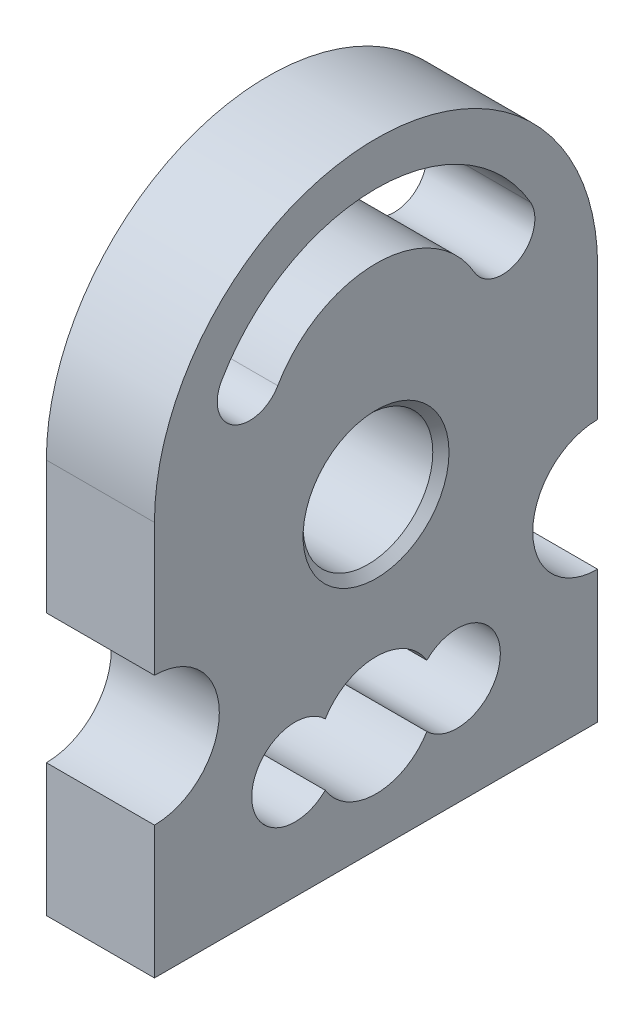
ISO-10303-21;
HEADER;
FILE_DESCRIPTION(('STEP AP214'),'2;1');
FILE_NAME('part.step','',(''),(''),'','','');
FILE_SCHEMA(('AUTOMOTIVE_DESIGN { 1 0 10303 214 1 1 1 1 }'));
ENDSEC;
DATA;
#1=APPLICATION_CONTEXT('core data for automotive mechanical design processes');
#2=APPLICATION_PROTOCOL_DEFINITION('international standard','automotive_design',2000,#1);
#3=PRODUCT_CONTEXT('',#1,'mechanical');
#4=PRODUCT('Part','Part','',(#3));
#5=PRODUCT_RELATED_PRODUCT_CATEGORY('part','',(#4));
#6=PRODUCT_DEFINITION_FORMATION('','',#4);
#7=PRODUCT_DEFINITION_CONTEXT('part definition',#1,'design');
#8=PRODUCT_DEFINITION('design','',#6,#7);
#9=PRODUCT_DEFINITION_SHAPE('','',#8);
#10=(LENGTH_UNIT() NAMED_UNIT(*) SI_UNIT(.MILLI.,.METRE.));
#11=(NAMED_UNIT(*) PLANE_ANGLE_UNIT() SI_UNIT($,.RADIAN.));
#12=(NAMED_UNIT(*) SI_UNIT($,.STERADIAN.) SOLID_ANGLE_UNIT());
#13=UNCERTAINTY_MEASURE_WITH_UNIT(LENGTH_MEASURE(1.E-05),#10,'distance_accuracy_value','');
#14=(GEOMETRIC_REPRESENTATION_CONTEXT(3) GLOBAL_UNCERTAINTY_ASSIGNED_CONTEXT((#13)) GLOBAL_UNIT_ASSIGNED_CONTEXT((#10,
#11,#12)) REPRESENTATION_CONTEXT('',''));
#15=CARTESIAN_POINT('',(0.,0.,0.));
#16=DIRECTION('',(0.,0.,1.));
#17=DIRECTION('',(1.,0.,0.));
#18=AXIS2_PLACEMENT_3D('',#15,#16,#17);
#19=CARTESIAN_POINT('',(20.,36.5,-41.));
#20=DIRECTION('',(1.,0.,0.));
#21=DIRECTION('',(0.,0.,-1.));
#22=AXIS2_PLACEMENT_3D('',#19,#20,#21);
#23=PLANE('',#22);
#24=CARTESIAN_POINT('',(20.,57.,0.));
#25=DIRECTION('',(1.,0.,0.));
#26=DIRECTION('',(0.,0.,-1.));
#27=AXIS2_PLACEMENT_3D('',#24,#25,#26);
#28=CIRCLE('',#27,13.5000000000001);
#29=CARTESIAN_POINT('',(20.,57.,-13.5000000000001));
#30=VERTEX_POINT('',#29);
#31=EDGE_CURVE('E11',#30,#30,#28,.F.);
#32=ORIENTED_EDGE('',*,*,#31,.T.);
#33=EDGE_LOOP('',(#32));
#34=FACE_BOUND('',#33,.T.);
#35=CARTESIAN_POINT('',(20.,20.,-15.));
#36=DIRECTION('',(1.,0.,0.));
#37=DIRECTION('',(0.,0.,-1.));
#38=AXIS2_PLACEMENT_3D('',#35,#36,#37);
#39=CIRCLE('',#38,8.);
#40=CARTESIAN_POINT('',(20.,14.2868572571657,-9.4));
#41=VERTEX_POINT('',#40);
#42=CARTESIAN_POINT('',(20.,25.7131427428343,-9.4));
#43=VERTEX_POINT('',#42);
#44=EDGE_CURVE('E193',#41,#43,#39,.T.);
#45=ORIENTED_EDGE('',*,*,#44,.F.);
#46=CARTESIAN_POINT('',(20.,20.,0.));
#47=DIRECTION('',(1.,0.,0.));
#48=DIRECTION('',(0.,0.,-1.));
#49=AXIS2_PLACEMENT_3D('',#46,#47,#48);
#50=CIRCLE('',#49,11.);
#51=CARTESIAN_POINT('',(20.,14.2868572571657,9.4));
#52=VERTEX_POINT('',#51);
#53=EDGE_CURVE('E192',#52,#41,#50,.T.);
#54=ORIENTED_EDGE('',*,*,#53,.F.);
#55=CARTESIAN_POINT('',(20.,20.,15.));
#56=DIRECTION('',(1.,0.,0.));
#57=DIRECTION('',(0.,0.,-1.));
#58=AXIS2_PLACEMENT_3D('',#55,#56,#57);
#59=CIRCLE('',#58,8.);
#60=CARTESIAN_POINT('',(20.,25.7131427428343,9.4));
#61=VERTEX_POINT('',#60);
#62=EDGE_CURVE('E200',#61,#52,#59,.T.);
#63=ORIENTED_EDGE('',*,*,#62,.F.);
#64=CARTESIAN_POINT('',(20.,20.,0.));
#65=DIRECTION('',(1.,0.,0.));
#66=DIRECTION('',(0.,0.,-1.));
#67=AXIS2_PLACEMENT_3D('',#64,#65,#66);
#68=CIRCLE('',#67,11.);
#69=EDGE_CURVE('E198',#43,#61,#68,.T.);
#70=ORIENTED_EDGE('',*,*,#69,.F.);
#71=EDGE_LOOP('',(#45,#54,#63,#70));
#72=FACE_BOUND('',#71,.T.);
#73=DIRECTION('',(0.,0.,-1.));
#74=VECTOR('',#73,1.);
#75=CARTESIAN_POINT('',(20.,0.,0.));
#76=LINE('',#75,#74);
#77=CARTESIAN_POINT('',(20.,0.,41.));
#78=VERTEX_POINT('',#77);
#79=CARTESIAN_POINT('',(20.,0.,-41.));
#80=VERTEX_POINT('',#79);
#81=EDGE_CURVE('E225',#78,#80,#76,.T.);
#82=ORIENTED_EDGE('',*,*,#81,.T.);
#83=DIRECTION('',(0.,1.,0.));
#84=VECTOR('',#83,1.);
#85=CARTESIAN_POINT('',(20.,24.5,-41.));
#86=LINE('',#85,#84);
#87=CARTESIAN_POINT('',(20.,24.5,-41.));
#88=VERTEX_POINT('',#87);
#89=EDGE_CURVE('E223',#80,#88,#86,.T.);
#90=ORIENTED_EDGE('',*,*,#89,.T.);
#91=CARTESIAN_POINT('',(20.,36.5,-41.));
#92=DIRECTION('',(-1.,0.,0.));
#93=DIRECTION('',(0.,0.,-1.));
#94=AXIS2_PLACEMENT_3D('',#91,#92,#93);
#95=CIRCLE('',#94,12.);
#96=CARTESIAN_POINT('',(20.,48.5,-41.));
#97=VERTEX_POINT('',#96);
#98=EDGE_CURVE('E229',#88,#97,#95,.T.);
#99=ORIENTED_EDGE('',*,*,#98,.T.);
#100=DIRECTION('',(0.,1.,0.));
#101=VECTOR('',#100,1.);
#102=CARTESIAN_POINT('',(20.,73.,-41.));
#103=LINE('',#102,#101);
#104=CARTESIAN_POINT('',(20.,73.,-41.));
#105=VERTEX_POINT('',#104);
#106=EDGE_CURVE('E228',#97,#105,#103,.T.);
#107=ORIENTED_EDGE('',*,*,#106,.T.);
#108=CARTESIAN_POINT('',(20.,73.,0.));
#109=DIRECTION('',(1.,0.,0.));
#110=DIRECTION('',(0.,0.,-1.));
#111=AXIS2_PLACEMENT_3D('',#108,#109,#110);
#112=CIRCLE('',#111,41.);
#113=CARTESIAN_POINT('',(20.,73.,41.));
#114=VERTEX_POINT('',#113);
#115=EDGE_CURVE('E235',#105,#114,#112,.T.);
#116=ORIENTED_EDGE('',*,*,#115,.T.);
#117=DIRECTION('',(0.,-1.,0.));
#118=VECTOR('',#117,1.);
#119=CARTESIAN_POINT('',(20.,73.,41.));
#120=LINE('',#119,#118);
#121=CARTESIAN_POINT('',(20.,48.5,41.));
#122=VERTEX_POINT('',#121);
#123=EDGE_CURVE('E234',#114,#122,#120,.T.);
#124=ORIENTED_EDGE('',*,*,#123,.T.);
#125=CARTESIAN_POINT('',(20.,36.5,41.));
#126=DIRECTION('',(-1.,0.,0.));
#127=DIRECTION('',(0.,0.,-1.));
#128=AXIS2_PLACEMENT_3D('',#125,#126,#127);
#129=CIRCLE('',#128,12.);
#130=CARTESIAN_POINT('',(20.,24.5,41.));
#131=VERTEX_POINT('',#130);
#132=EDGE_CURVE('E237',#122,#131,#129,.T.);
#133=ORIENTED_EDGE('',*,*,#132,.T.);
#134=DIRECTION('',(0.,-1.,0.));
#135=VECTOR('',#134,1.);
#136=CARTESIAN_POINT('',(20.,24.5,41.));
#137=LINE('',#136,#135);
#138=EDGE_CURVE('E236',#131,#78,#137,.T.);
#139=ORIENTED_EDGE('',*,*,#138,.T.);
#140=EDGE_LOOP('',(#82,#90,#99,#107,#116,#124,#133,#139));
#141=FACE_BOUND('',#140,.T.);
#142=CARTESIAN_POINT('',(20.,73.,0.));
#143=DIRECTION('',(1.,0.,0.));
#144=DIRECTION('',(0.,0.,-1.));
#145=AXIS2_PLACEMENT_3D('',#142,#143,#144);
#146=CIRCLE('',#145,33.);
#147=CARTESIAN_POINT('',(20.,89.4999999999999,-28.5788383248865));
#148=VERTEX_POINT('',#147);
#149=CARTESIAN_POINT('',(20.,89.4999999999999,28.5788383248865));
#150=VERTEX_POINT('',#149);
#151=EDGE_CURVE('E162',#148,#150,#146,.T.);
#152=ORIENTED_EDGE('',*,*,#151,.F.);
#153=CARTESIAN_POINT('',(20.,86.4999999999999,-23.3826859021799));
#154=DIRECTION('',(1.,0.,0.));
#155=DIRECTION('',(0.,0.,-1.));
#156=AXIS2_PLACEMENT_3D('',#153,#154,#155);
#157=CIRCLE('',#156,6.);
#158=CARTESIAN_POINT('',(20.,83.4999999999999,-18.1865334794732));
#159=VERTEX_POINT('',#158);
#160=EDGE_CURVE('E154',#159,#148,#157,.T.);
#161=ORIENTED_EDGE('',*,*,#160,.F.);
#162=CARTESIAN_POINT('',(20.,73.,0.));
#163=DIRECTION('',(-1.,0.,0.));
#164=DIRECTION('',(0.,0.,-1.));
#165=AXIS2_PLACEMENT_3D('',#162,#163,#164);
#166=CIRCLE('',#165,21.);
#167=CARTESIAN_POINT('',(20.,83.4999999999999,18.1865334794732));
#168=VERTEX_POINT('',#167);
#169=EDGE_CURVE('E180',#168,#159,#166,.T.);
#170=ORIENTED_EDGE('',*,*,#169,.F.);
#171=CARTESIAN_POINT('',(20.,86.4999999999999,23.3826859021799));
#172=DIRECTION('',(1.,0.,0.));
#173=DIRECTION('',(0.,0.,-1.));
#174=AXIS2_PLACEMENT_3D('',#171,#172,#173);
#175=CIRCLE('',#174,6.);
#176=EDGE_CURVE('E173',#150,#168,#175,.T.);
#177=ORIENTED_EDGE('',*,*,#176,.F.);
#178=EDGE_LOOP('',(#152,#161,#170,#177));
#179=FACE_BOUND('',#178,.T.);
#180=ADVANCED_FACE('F41',(#34,#72,#141,#179),#23,.T.);
#181=CARTESIAN_POINT('',(0.,36.5,-41.));
#182=DIRECTION('',(1.,0.,0.));
#183=DIRECTION('',(0.,0.,-1.));
#184=AXIS2_PLACEMENT_3D('',#181,#182,#183);
#185=PLANE('',#184);
#186=CARTESIAN_POINT('',(0.,57.,0.));
#187=DIRECTION('',(1.,0.,0.));
#188=DIRECTION('',(0.,0.,-1.));
#189=AXIS2_PLACEMENT_3D('',#186,#187,#188);
#190=CIRCLE('',#189,13.5);
#191=CARTESIAN_POINT('',(0.,57.,-13.5));
#192=VERTEX_POINT('',#191);
#193=EDGE_CURVE('E276',#192,#192,#190,.T.);
#194=ORIENTED_EDGE('',*,*,#193,.T.);
#195=EDGE_LOOP('',(#194));
#196=FACE_BOUND('',#195,.T.);
#197=CARTESIAN_POINT('',(0.,20.,0.));
#198=DIRECTION('',(1.,0.,0.));
#199=DIRECTION('',(0.,0.,-1.));
#200=AXIS2_PLACEMENT_3D('',#197,#198,#199);
#201=CIRCLE('',#200,11.);
#202=CARTESIAN_POINT('',(0.,14.2868572571657,9.4));
#203=VERTEX_POINT('',#202);
#204=CARTESIAN_POINT('',(0.,14.2868572571657,-9.4));
#205=VERTEX_POINT('',#204);
#206=EDGE_CURVE('E172',#203,#205,#201,.T.);
#207=ORIENTED_EDGE('',*,*,#206,.T.);
#208=CARTESIAN_POINT('',(0.,20.,-15.));
#209=DIRECTION('',(1.,0.,0.));
#210=DIRECTION('',(0.,0.,-1.));
#211=AXIS2_PLACEMENT_3D('',#208,#209,#210);
#212=CIRCLE('',#211,8.);
#213=CARTESIAN_POINT('',(0.,25.7131427428343,-9.4));
#214=VERTEX_POINT('',#213);
#215=EDGE_CURVE('E204',#205,#214,#212,.T.);
#216=ORIENTED_EDGE('',*,*,#215,.T.);
#217=CARTESIAN_POINT('',(0.,20.,0.));
#218=DIRECTION('',(1.,0.,0.));
#219=DIRECTION('',(0.,0.,-1.));
#220=AXIS2_PLACEMENT_3D('',#217,#218,#219);
#221=CIRCLE('',#220,11.);
#222=CARTESIAN_POINT('',(0.,25.7131427428343,9.4));
#223=VERTEX_POINT('',#222);
#224=EDGE_CURVE('E210',#214,#223,#221,.T.);
#225=ORIENTED_EDGE('',*,*,#224,.T.);
#226=CARTESIAN_POINT('',(0.,20.,15.));
#227=DIRECTION('',(1.,0.,0.));
#228=DIRECTION('',(0.,0.,-1.));
#229=AXIS2_PLACEMENT_3D('',#226,#227,#228);
#230=CIRCLE('',#229,8.);
#231=EDGE_CURVE('E194',#223,#203,#230,.T.);
#232=ORIENTED_EDGE('',*,*,#231,.T.);
#233=EDGE_LOOP('',(#207,#216,#225,#232));
#234=FACE_BOUND('',#233,.T.);
#235=DIRECTION('',(0.,1.,0.));
#236=VECTOR('',#235,1.);
#237=CARTESIAN_POINT('',(0.,24.5,-41.));
#238=LINE('',#237,#236);
#239=CARTESIAN_POINT('',(0.,0.,-41.));
#240=VERTEX_POINT('',#239);
#241=CARTESIAN_POINT('',(0.,24.5,-41.));
#242=VERTEX_POINT('',#241);
#243=EDGE_CURVE('E222',#240,#242,#238,.T.);
#244=ORIENTED_EDGE('',*,*,#243,.F.);
#245=DIRECTION('',(0.,0.,-1.));
#246=VECTOR('',#245,1.);
#247=CARTESIAN_POINT('',(0.,0.,0.));
#248=LINE('',#247,#246);
#249=CARTESIAN_POINT('',(0.,0.,41.));
#250=VERTEX_POINT('',#249);
#251=EDGE_CURVE('E227',#250,#240,#248,.T.);
#252=ORIENTED_EDGE('',*,*,#251,.F.);
#253=DIRECTION('',(0.,-1.,0.));
#254=VECTOR('',#253,1.);
#255=CARTESIAN_POINT('',(0.,24.5,41.));
#256=LINE('',#255,#254);
#257=CARTESIAN_POINT('',(0.,24.5,41.));
#258=VERTEX_POINT('',#257);
#259=EDGE_CURVE('E251',#258,#250,#256,.T.);
#260=ORIENTED_EDGE('',*,*,#259,.F.);
#261=CARTESIAN_POINT('',(0.,36.5,41.));
#262=DIRECTION('',(-1.,0.,0.));
#263=DIRECTION('',(0.,0.,-1.));
#264=AXIS2_PLACEMENT_3D('',#261,#262,#263);
#265=CIRCLE('',#264,12.);
#266=CARTESIAN_POINT('',(0.,48.5,41.));
#267=VERTEX_POINT('',#266);
#268=EDGE_CURVE('E253',#267,#258,#265,.T.);
#269=ORIENTED_EDGE('',*,*,#268,.F.);
#270=DIRECTION('',(0.,-1.,0.));
#271=VECTOR('',#270,1.);
#272=CARTESIAN_POINT('',(0.,73.,41.));
#273=LINE('',#272,#271);
#274=CARTESIAN_POINT('',(0.,73.,41.));
#275=VERTEX_POINT('',#274);
#276=EDGE_CURVE('E249',#275,#267,#273,.T.);
#277=ORIENTED_EDGE('',*,*,#276,.F.);
#278=CARTESIAN_POINT('',(0.,73.,0.));
#279=DIRECTION('',(1.,0.,0.));
#280=DIRECTION('',(0.,0.,-1.));
#281=AXIS2_PLACEMENT_3D('',#278,#279,#280);
#282=CIRCLE('',#281,41.);
#283=CARTESIAN_POINT('',(0.,73.,-41.));
#284=VERTEX_POINT('',#283);
#285=EDGE_CURVE('E250',#284,#275,#282,.T.);
#286=ORIENTED_EDGE('',*,*,#285,.F.);
#287=DIRECTION('',(0.,1.,0.));
#288=VECTOR('',#287,1.);
#289=CARTESIAN_POINT('',(0.,73.,-41.));
#290=LINE('',#289,#288);
#291=CARTESIAN_POINT('',(0.,48.5,-41.));
#292=VERTEX_POINT('',#291);
#293=EDGE_CURVE('E243',#292,#284,#290,.T.);
#294=ORIENTED_EDGE('',*,*,#293,.F.);
#295=CARTESIAN_POINT('',(0.,36.5,-41.));
#296=DIRECTION('',(-1.,0.,0.));
#297=DIRECTION('',(0.,0.,-1.));
#298=AXIS2_PLACEMENT_3D('',#295,#296,#297);
#299=CIRCLE('',#298,12.);
#300=EDGE_CURVE('E244',#242,#292,#299,.T.);
#301=ORIENTED_EDGE('',*,*,#300,.F.);
#302=EDGE_LOOP('',(#244,#252,#260,#269,#277,#286,#294,#301));
#303=FACE_BOUND('',#302,.T.);
#304=CARTESIAN_POINT('',(0.,86.4999999999999,-23.3826859021799));
#305=DIRECTION('',(1.,0.,0.));
#306=DIRECTION('',(0.,0.,-1.));
#307=AXIS2_PLACEMENT_3D('',#304,#305,#306);
#308=CIRCLE('',#307,6.);
#309=CARTESIAN_POINT('',(0.,83.4999999999999,-18.1865334794732));
#310=VERTEX_POINT('',#309);
#311=CARTESIAN_POINT('',(0.,89.4999999999999,-28.5788383248865));
#312=VERTEX_POINT('',#311);
#313=EDGE_CURVE('E63',#310,#312,#308,.T.);
#314=ORIENTED_EDGE('',*,*,#313,.T.);
#315=CARTESIAN_POINT('',(0.,73.,0.));
#316=DIRECTION('',(1.,0.,0.));
#317=DIRECTION('',(0.,0.,-1.));
#318=AXIS2_PLACEMENT_3D('',#315,#316,#317);
#319=CIRCLE('',#318,33.);
#320=CARTESIAN_POINT('',(0.,89.4999999999999,28.5788383248865));
#321=VERTEX_POINT('',#320);
#322=EDGE_CURVE('E168',#312,#321,#319,.T.);
#323=ORIENTED_EDGE('',*,*,#322,.T.);
#324=CARTESIAN_POINT('',(0.,86.4999999999999,23.3826859021799));
#325=DIRECTION('',(1.,0.,0.));
#326=DIRECTION('',(0.,0.,-1.));
#327=AXIS2_PLACEMENT_3D('',#324,#325,#326);
#328=CIRCLE('',#327,6.);
#329=CARTESIAN_POINT('',(0.,83.4999999999999,18.1865334794733));
#330=VERTEX_POINT('',#329);
#331=EDGE_CURVE('E181',#321,#330,#328,.T.);
#332=ORIENTED_EDGE('',*,*,#331,.T.);
#333=CARTESIAN_POINT('',(0.,73.,0.));
#334=DIRECTION('',(-1.,0.,0.));
#335=DIRECTION('',(0.,0.,-1.));
#336=AXIS2_PLACEMENT_3D('',#333,#334,#335);
#337=CIRCLE('',#336,21.);
#338=EDGE_CURVE('E163',#330,#310,#337,.T.);
#339=ORIENTED_EDGE('',*,*,#338,.T.);
#340=EDGE_LOOP('',(#314,#323,#332,#339));
#341=FACE_BOUND('',#340,.T.);
#342=ADVANCED_FACE('F297',(#196,#234,#303,#341),#185,.F.);
#343=CARTESIAN_POINT('',(20.,24.5,-41.));
#344=DIRECTION('',(0.,0.,1.));
#345=DIRECTION('',(1.,0.,0.));
#346=AXIS2_PLACEMENT_3D('',#343,#344,#345);
#347=PLANE('',#346);
#348=ORIENTED_EDGE('',*,*,#243,.T.);
#349=DIRECTION('',(-1.,0.,0.));
#350=VECTOR('',#349,1.);
#351=CARTESIAN_POINT('',(20.,24.5,-41.));
#352=LINE('',#351,#350);
#353=EDGE_CURVE('E272',#88,#242,#352,.T.);
#354=ORIENTED_EDGE('',*,*,#353,.F.);
#355=ORIENTED_EDGE('',*,*,#89,.F.);
#356=DIRECTION('',(-1.,0.,0.));
#357=VECTOR('',#356,1.);
#358=CARTESIAN_POINT('',(20.,0.,-41.));
#359=LINE('',#358,#357);
#360=EDGE_CURVE('E277',#80,#240,#359,.T.);
#361=ORIENTED_EDGE('',*,*,#360,.T.);
#362=EDGE_LOOP('',(#348,#354,#355,#361));
#363=FACE_BOUND('',#362,.T.);
#364=ADVANCED_FACE('F296',(#363),#347,.F.);
#365=CARTESIAN_POINT('',(20.,36.5,-41.));
#366=DIRECTION('',(-1.,0.,0.));
#367=DIRECTION('',(0.,0.,1.));
#368=AXIS2_PLACEMENT_3D('',#365,#366,#367);
#369=CYLINDRICAL_SURFACE('',#368,12.);
#370=ORIENTED_EDGE('',*,*,#300,.T.);
#371=DIRECTION('',(-1.,0.,0.));
#372=VECTOR('',#371,1.);
#373=CARTESIAN_POINT('',(20.,48.5,-41.));
#374=LINE('',#373,#372);
#375=EDGE_CURVE('E269',#97,#292,#374,.T.);
#376=ORIENTED_EDGE('',*,*,#375,.F.);
#377=ORIENTED_EDGE('',*,*,#98,.F.);
#378=ORIENTED_EDGE('',*,*,#353,.T.);
#379=EDGE_LOOP('',(#370,#376,#377,#378));
#380=FACE_BOUND('',#379,.T.);
#381=ADVANCED_FACE('F346',(#380),#369,.F.);
#382=CARTESIAN_POINT('',(20.,73.,-41.));
#383=DIRECTION('',(0.,0.,1.));
#384=DIRECTION('',(1.,0.,0.));
#385=AXIS2_PLACEMENT_3D('',#382,#383,#384);
#386=PLANE('',#385);
#387=ORIENTED_EDGE('',*,*,#293,.T.);
#388=DIRECTION('',(-1.,0.,0.));
#389=VECTOR('',#388,1.);
#390=CARTESIAN_POINT('',(20.,73.,-41.));
#391=LINE('',#390,#389);
#392=EDGE_CURVE('E270',#105,#284,#391,.T.);
#393=ORIENTED_EDGE('',*,*,#392,.F.);
#394=ORIENTED_EDGE('',*,*,#106,.F.);
#395=ORIENTED_EDGE('',*,*,#375,.T.);
#396=EDGE_LOOP('',(#387,#393,#394,#395));
#397=FACE_BOUND('',#396,.T.);
#398=ADVANCED_FACE('F344',(#397),#386,.F.);
#399=CARTESIAN_POINT('',(20.,73.,0.));
#400=DIRECTION('',(-1.,0.,0.));
#401=DIRECTION('',(0.,0.,1.));
#402=AXIS2_PLACEMENT_3D('',#399,#400,#401);
#403=CYLINDRICAL_SURFACE('',#402,41.);
#404=ORIENTED_EDGE('',*,*,#285,.T.);
#405=DIRECTION('',(-1.,0.,0.));
#406=VECTOR('',#405,1.);
#407=CARTESIAN_POINT('',(20.,73.,41.));
#408=LINE('',#407,#406);
#409=EDGE_CURVE('E262',#114,#275,#408,.T.);
#410=ORIENTED_EDGE('',*,*,#409,.F.);
#411=ORIENTED_EDGE('',*,*,#115,.F.);
#412=ORIENTED_EDGE('',*,*,#392,.T.);
#413=EDGE_LOOP('',(#404,#410,#411,#412));
#414=FACE_BOUND('',#413,.T.);
#415=ADVANCED_FACE('F338',(#414),#403,.T.);
#416=CARTESIAN_POINT('',(20.,73.,41.));
#417=DIRECTION('',(0.,0.,-1.));
#418=DIRECTION('',(-1.,0.,0.));
#419=AXIS2_PLACEMENT_3D('',#416,#417,#418);
#420=PLANE('',#419);
#421=ORIENTED_EDGE('',*,*,#276,.T.);
#422=DIRECTION('',(-1.,0.,0.));
#423=VECTOR('',#422,1.);
#424=CARTESIAN_POINT('',(20.,48.5,41.));
#425=LINE('',#424,#423);
#426=EDGE_CURVE('E261',#122,#267,#425,.T.);
#427=ORIENTED_EDGE('',*,*,#426,.F.);
#428=ORIENTED_EDGE('',*,*,#123,.F.);
#429=ORIENTED_EDGE('',*,*,#409,.T.);
#430=EDGE_LOOP('',(#421,#427,#428,#429));
#431=FACE_BOUND('',#430,.T.);
#432=ADVANCED_FACE('F337',(#431),#420,.F.);
#433=CARTESIAN_POINT('',(20.,36.5,41.));
#434=DIRECTION('',(-1.,0.,0.));
#435=DIRECTION('',(0.,0.,1.));
#436=AXIS2_PLACEMENT_3D('',#433,#434,#435);
#437=CYLINDRICAL_SURFACE('',#436,12.);
#438=ORIENTED_EDGE('',*,*,#268,.T.);
#439=DIRECTION('',(-1.,0.,0.));
#440=VECTOR('',#439,1.);
#441=CARTESIAN_POINT('',(20.,24.5,41.));
#442=LINE('',#441,#440);
#443=EDGE_CURVE('E256',#131,#258,#442,.T.);
#444=ORIENTED_EDGE('',*,*,#443,.F.);
#445=ORIENTED_EDGE('',*,*,#132,.F.);
#446=ORIENTED_EDGE('',*,*,#426,.T.);
#447=EDGE_LOOP('',(#438,#444,#445,#446));
#448=FACE_BOUND('',#447,.T.);
#449=ADVANCED_FACE('F335',(#448),#437,.F.);
#450=CARTESIAN_POINT('',(20.,24.5,41.));
#451=DIRECTION('',(0.,0.,-1.));
#452=DIRECTION('',(-1.,0.,0.));
#453=AXIS2_PLACEMENT_3D('',#450,#451,#452);
#454=PLANE('',#453);
#455=ORIENTED_EDGE('',*,*,#259,.T.);
#456=DIRECTION('',(-1.,0.,0.));
#457=VECTOR('',#456,1.);
#458=CARTESIAN_POINT('',(20.,0.,41.));
#459=LINE('',#458,#457);
#460=EDGE_CURVE('E242',#78,#250,#459,.T.);
#461=ORIENTED_EDGE('',*,*,#460,.F.);
#462=ORIENTED_EDGE('',*,*,#138,.F.);
#463=ORIENTED_EDGE('',*,*,#443,.T.);
#464=EDGE_LOOP('',(#455,#461,#462,#463));
#465=FACE_BOUND('',#464,.T.);
#466=ADVANCED_FACE('F327',(#465),#454,.F.);
#467=CARTESIAN_POINT('',(20.,0.,0.));
#468=DIRECTION('',(0.,1.,0.));
#469=DIRECTION('',(0.,0.,1.));
#470=AXIS2_PLACEMENT_3D('',#467,#468,#469);
#471=PLANE('',#470);
#472=ORIENTED_EDGE('',*,*,#251,.T.);
#473=ORIENTED_EDGE('',*,*,#360,.F.);
#474=ORIENTED_EDGE('',*,*,#81,.F.);
#475=ORIENTED_EDGE('',*,*,#460,.T.);
#476=EDGE_LOOP('',(#472,#473,#474,#475));
#477=FACE_BOUND('',#476,.T.);
#478=ADVANCED_FACE('F324',(#477),#471,.F.);
#479=CARTESIAN_POINT('',(20.,20.,0.));
#480=DIRECTION('',(-1.,0.,0.));
#481=DIRECTION('',(0.,0.,1.));
#482=AXIS2_PLACEMENT_3D('',#479,#480,#481);
#483=CYLINDRICAL_SURFACE('',#482,11.);
#484=ORIENTED_EDGE('',*,*,#206,.F.);
#485=DIRECTION('',(-1.,0.,0.));
#486=VECTOR('',#485,1.);
#487=CARTESIAN_POINT('',(20.,14.2868572571657,9.4));
#488=LINE('',#487,#486);
#489=EDGE_CURVE('E203',#52,#203,#488,.T.);
#490=ORIENTED_EDGE('',*,*,#489,.F.);
#491=ORIENTED_EDGE('',*,*,#53,.T.);
#492=DIRECTION('',(-1.,0.,0.));
#493=VECTOR('',#492,1.);
#494=CARTESIAN_POINT('',(20.,14.2868572571657,-9.4));
#495=LINE('',#494,#493);
#496=EDGE_CURVE('E217',#41,#205,#495,.T.);
#497=ORIENTED_EDGE('',*,*,#496,.T.);
#498=EDGE_LOOP('',(#484,#490,#491,#497));
#499=FACE_BOUND('',#498,.T.);
#500=ADVANCED_FACE('F325',(#499),#483,.F.);
#501=CARTESIAN_POINT('',(20.,20.,-15.));
#502=DIRECTION('',(-1.,0.,0.));
#503=DIRECTION('',(0.,0.,1.));
#504=AXIS2_PLACEMENT_3D('',#501,#502,#503);
#505=CYLINDRICAL_SURFACE('',#504,8.);
#506=ORIENTED_EDGE('',*,*,#215,.F.);
#507=ORIENTED_EDGE('',*,*,#496,.F.);
#508=ORIENTED_EDGE('',*,*,#44,.T.);
#509=DIRECTION('',(-1.,0.,0.));
#510=VECTOR('',#509,1.);
#511=CARTESIAN_POINT('',(20.,25.7131427428343,-9.4));
#512=LINE('',#511,#510);
#513=EDGE_CURVE('E216',#43,#214,#512,.T.);
#514=ORIENTED_EDGE('',*,*,#513,.T.);
#515=EDGE_LOOP('',(#506,#507,#508,#514));
#516=FACE_BOUND('',#515,.T.);
#517=ADVANCED_FACE('F422',(#516),#505,.F.);
#518=CARTESIAN_POINT('',(20.,20.,0.));
#519=DIRECTION('',(-1.,0.,0.));
#520=DIRECTION('',(0.,0.,1.));
#521=AXIS2_PLACEMENT_3D('',#518,#519,#520);
#522=CYLINDRICAL_SURFACE('',#521,11.);
#523=ORIENTED_EDGE('',*,*,#224,.F.);
#524=ORIENTED_EDGE('',*,*,#513,.F.);
#525=ORIENTED_EDGE('',*,*,#69,.T.);
#526=DIRECTION('',(-1.,0.,0.));
#527=VECTOR('',#526,1.);
#528=CARTESIAN_POINT('',(20.,25.7131427428343,9.4));
#529=LINE('',#528,#527);
#530=EDGE_CURVE('E212',#61,#223,#529,.T.);
#531=ORIENTED_EDGE('',*,*,#530,.T.);
#532=EDGE_LOOP('',(#523,#524,#525,#531));
#533=FACE_BOUND('',#532,.T.);
#534=ADVANCED_FACE('F433',(#533),#522,.F.);
#535=CARTESIAN_POINT('',(20.,20.,15.));
#536=DIRECTION('',(-1.,0.,0.));
#537=DIRECTION('',(0.,0.,1.));
#538=AXIS2_PLACEMENT_3D('',#535,#536,#537);
#539=CYLINDRICAL_SURFACE('',#538,8.);
#540=ORIENTED_EDGE('',*,*,#231,.F.);
#541=ORIENTED_EDGE('',*,*,#530,.F.);
#542=ORIENTED_EDGE('',*,*,#62,.T.);
#543=ORIENTED_EDGE('',*,*,#489,.T.);
#544=EDGE_LOOP('',(#540,#541,#542,#543));
#545=FACE_BOUND('',#544,.T.);
#546=ADVANCED_FACE('F442',(#545),#539,.F.);
#547=CARTESIAN_POINT('',(20.,57.,0.));
#548=DIRECTION('',(-1.,0.,0.));
#549=DIRECTION('',(0.,0.,1.));
#550=AXIS2_PLACEMENT_3D('',#547,#548,#549);
#551=CYLINDRICAL_SURFACE('',#550,12.);
#552=CARTESIAN_POINT('',(1.50000000000002,57.,0.));
#553=DIRECTION('',(1.,0.,0.));
#554=DIRECTION('',(0.,0.,-1.));
#555=AXIS2_PLACEMENT_3D('',#552,#553,#554);
#556=CIRCLE('',#555,12.);
#557=CARTESIAN_POINT('',(1.50000000000002,57.,-12.));
#558=VERTEX_POINT('',#557);
#559=EDGE_CURVE('E49',#558,#558,#556,.F.);
#560=ORIENTED_EDGE('',*,*,#559,.T.);
#561=EDGE_LOOP('',(#560));
#562=FACE_BOUND('',#561,.T.);
#563=CARTESIAN_POINT('',(18.5,57.,0.));
#564=DIRECTION('',(1.,0.,0.));
#565=DIRECTION('',(0.,0.,-1.));
#566=AXIS2_PLACEMENT_3D('',#563,#564,#565);
#567=CIRCLE('',#566,12.);
#568=CARTESIAN_POINT('',(18.5,57.,-12.));
#569=VERTEX_POINT('',#568);
#570=EDGE_CURVE('E285',#569,#569,#567,.T.);
#571=ORIENTED_EDGE('',*,*,#570,.T.);
#572=EDGE_LOOP('',(#571));
#573=FACE_BOUND('',#572,.T.);
#574=ADVANCED_FACE('F290',(#562,#573),#551,.F.);
#575=CARTESIAN_POINT('',(20.,86.4999999999999,-23.3826859021799));
#576=DIRECTION('',(-1.,0.,0.));
#577=DIRECTION('',(0.,0.,1.));
#578=AXIS2_PLACEMENT_3D('',#575,#576,#577);
#579=CYLINDRICAL_SURFACE('',#578,6.);
#580=ORIENTED_EDGE('',*,*,#313,.F.);
#581=DIRECTION('',(-1.,0.,0.));
#582=VECTOR('',#581,1.);
#583=CARTESIAN_POINT('',(20.,83.4999999999999,-18.1865334794732));
#584=LINE('',#583,#582);
#585=EDGE_CURVE('E157',#159,#310,#584,.T.);
#586=ORIENTED_EDGE('',*,*,#585,.F.);
#587=ORIENTED_EDGE('',*,*,#160,.T.);
#588=DIRECTION('',(-1.,0.,0.));
#589=VECTOR('',#588,1.);
#590=CARTESIAN_POINT('',(20.,89.4999999999999,-28.5788383248865));
#591=LINE('',#590,#589);
#592=EDGE_CURVE('E158',#148,#312,#591,.T.);
#593=ORIENTED_EDGE('',*,*,#592,.T.);
#594=EDGE_LOOP('',(#580,#586,#587,#593));
#595=FACE_BOUND('',#594,.T.);
#596=ADVANCED_FACE('F160',(#595),#579,.F.);
#597=CARTESIAN_POINT('',(20.,73.,0.));
#598=DIRECTION('',(-1.,0.,0.));
#599=DIRECTION('',(0.,0.,1.));
#600=AXIS2_PLACEMENT_3D('',#597,#598,#599);
#601=CYLINDRICAL_SURFACE('',#600,33.);
#602=ORIENTED_EDGE('',*,*,#322,.F.);
#603=ORIENTED_EDGE('',*,*,#592,.F.);
#604=ORIENTED_EDGE('',*,*,#151,.T.);
#605=DIRECTION('',(-1.,0.,0.));
#606=VECTOR('',#605,1.);
#607=CARTESIAN_POINT('',(20.,89.4999999999999,28.5788383248865));
#608=LINE('',#607,#606);
#609=EDGE_CURVE('E175',#150,#321,#608,.T.);
#610=ORIENTED_EDGE('',*,*,#609,.T.);
#611=EDGE_LOOP('',(#602,#603,#604,#610));
#612=FACE_BOUND('',#611,.T.);
#613=ADVANCED_FACE('F170',(#612),#601,.F.);
#614=CARTESIAN_POINT('',(20.,86.4999999999999,23.3826859021799));
#615=DIRECTION('',(-1.,0.,0.));
#616=DIRECTION('',(0.,0.,1.));
#617=AXIS2_PLACEMENT_3D('',#614,#615,#616);
#618=CYLINDRICAL_SURFACE('',#617,6.);
#619=ORIENTED_EDGE('',*,*,#331,.F.);
#620=ORIENTED_EDGE('',*,*,#609,.F.);
#621=ORIENTED_EDGE('',*,*,#176,.T.);
#622=DIRECTION('',(-1.,0.,0.));
#623=VECTOR('',#622,1.);
#624=CARTESIAN_POINT('',(20.,83.4999999999999,18.1865334794733));
#625=LINE('',#624,#623);
#626=EDGE_CURVE('E60',#168,#330,#625,.T.);
#627=ORIENTED_EDGE('',*,*,#626,.T.);
#628=EDGE_LOOP('',(#619,#620,#621,#627));
#629=FACE_BOUND('',#628,.T.);
#630=ADVANCED_FACE('F306',(#629),#618,.F.);
#631=CARTESIAN_POINT('',(20.,73.,0.));
#632=DIRECTION('',(-1.,0.,0.));
#633=DIRECTION('',(0.,0.,1.));
#634=AXIS2_PLACEMENT_3D('',#631,#632,#633);
#635=CYLINDRICAL_SURFACE('',#634,21.);
#636=ORIENTED_EDGE('',*,*,#338,.F.);
#637=ORIENTED_EDGE('',*,*,#626,.F.);
#638=ORIENTED_EDGE('',*,*,#169,.T.);
#639=ORIENTED_EDGE('',*,*,#585,.T.);
#640=EDGE_LOOP('',(#636,#637,#638,#639));
#641=FACE_BOUND('',#640,.T.);
#642=ADVANCED_FACE('F291',(#641),#635,.T.);
#643=CARTESIAN_POINT('',(0.,57.,0.));
#644=DIRECTION('',(-1.,0.,0.));
#645=DIRECTION('',(0.,0.,1.));
#646=AXIS2_PLACEMENT_3D('',#643,#644,#645);
#647=CONICAL_SURFACE('',#646,13.5,0.785398163397444);
#648=ORIENTED_EDGE('',*,*,#559,.F.);
#649=EDGE_LOOP('',(#648));
#650=FACE_BOUND('',#649,.T.);
#651=ORIENTED_EDGE('',*,*,#193,.F.);
#652=EDGE_LOOP('',(#651));
#653=FACE_BOUND('',#652,.T.);
#654=ADVANCED_FACE('F286',(#650,#653),#647,.F.);
#655=CARTESIAN_POINT('',(18.5,57.,0.));
#656=DIRECTION('',(1.,0.,0.));
#657=DIRECTION('',(0.,0.,-1.));
#658=AXIS2_PLACEMENT_3D('',#655,#656,#657);
#659=CONICAL_SURFACE('',#658,12.,0.785398163397454);
#660=CARTESIAN_POINT('',(20.,57.,-13.5000000000001));
#661=CARTESIAN_POINT('',(19.984375,57.,-13.484375));
#662=CARTESIAN_POINT('',(19.96875,57.,-13.46875));
#663=CARTESIAN_POINT('',(19.9375,57.,-13.4375));
#664=CARTESIAN_POINT('',(19.921875,57.,-13.421875));
#665=CARTESIAN_POINT('',(19.890625,57.,-13.390625));
#666=CARTESIAN_POINT('',(19.875,57.,-13.375));
#667=CARTESIAN_POINT('',(19.84375,57.,-13.34375));
#668=CARTESIAN_POINT('',(19.828125,57.,-13.328125));
#669=CARTESIAN_POINT('',(19.796875,57.,-13.296875));
#670=CARTESIAN_POINT('',(19.78125,57.,-13.28125));
#671=CARTESIAN_POINT('',(19.75,57.,-13.25));
#672=CARTESIAN_POINT('',(19.734375,57.,-13.234375));
#673=CARTESIAN_POINT('',(19.703125,57.,-13.203125));
#674=CARTESIAN_POINT('',(19.6875,57.,-13.1875));
#675=CARTESIAN_POINT('',(19.65625,57.,-13.15625));
#676=CARTESIAN_POINT('',(19.640625,57.,-13.140625));
#677=CARTESIAN_POINT('',(19.609375,57.,-13.109375));
#678=CARTESIAN_POINT('',(19.59375,57.,-13.09375));
#679=CARTESIAN_POINT('',(19.5625,57.,-13.0625));
#680=CARTESIAN_POINT('',(19.546875,57.,-13.046875));
#681=CARTESIAN_POINT('',(19.515625,57.,-13.015625));
#682=CARTESIAN_POINT('',(19.5,57.,-13.));
#683=CARTESIAN_POINT('',(19.46875,57.,-12.96875));
#684=CARTESIAN_POINT('',(19.453125,57.,-12.953125));
#685=CARTESIAN_POINT('',(19.421875,57.,-12.921875));
#686=CARTESIAN_POINT('',(19.40625,57.,-12.90625));
#687=CARTESIAN_POINT('',(19.375,57.,-12.875));
#688=CARTESIAN_POINT('',(19.359375,57.,-12.859375));
#689=CARTESIAN_POINT('',(19.328125,57.,-12.828125));
#690=CARTESIAN_POINT('',(19.3125,57.,-12.8125));
#691=CARTESIAN_POINT('',(19.28125,57.,-12.78125));
#692=CARTESIAN_POINT('',(19.265625,57.,-12.765625));
#693=CARTESIAN_POINT('',(19.234375,57.,-12.734375));
#694=CARTESIAN_POINT('',(19.21875,57.,-12.71875));
#695=CARTESIAN_POINT('',(19.1875,57.,-12.6875));
#696=CARTESIAN_POINT('',(19.171875,57.,-12.671875));
#697=CARTESIAN_POINT('',(19.140625,57.,-12.640625));
#698=CARTESIAN_POINT('',(19.125,57.,-12.625));
#699=CARTESIAN_POINT('',(19.09375,57.,-12.59375));
#700=CARTESIAN_POINT('',(19.078125,57.,-12.578125));
#701=CARTESIAN_POINT('',(19.046875,57.,-12.546875));
#702=CARTESIAN_POINT('',(19.03125,57.,-12.53125));
#703=CARTESIAN_POINT('',(19.,57.,-12.5));
#704=CARTESIAN_POINT('',(18.984375,57.,-12.484375));
#705=CARTESIAN_POINT('',(18.953125,57.,-12.453125));
#706=CARTESIAN_POINT('',(18.9375,57.,-12.4375));
#707=CARTESIAN_POINT('',(18.90625,57.,-12.40625));
#708=CARTESIAN_POINT('',(18.890625,57.,-12.390625));
#709=CARTESIAN_POINT('',(18.859375,57.,-12.359375));
#710=CARTESIAN_POINT('',(18.84375,57.,-12.34375));
#711=CARTESIAN_POINT('',(18.8125,57.,-12.3125));
#712=CARTESIAN_POINT('',(18.796875,57.,-12.296875));
#713=CARTESIAN_POINT('',(18.765625,57.,-12.265625));
#714=CARTESIAN_POINT('',(18.75,57.,-12.25));
#715=CARTESIAN_POINT('',(18.71875,57.,-12.21875));
#716=CARTESIAN_POINT('',(18.703125,57.,-12.203125));
#717=CARTESIAN_POINT('',(18.671875,57.,-12.171875));
#718=CARTESIAN_POINT('',(18.65625,57.,-12.15625));
#719=CARTESIAN_POINT('',(18.625,57.,-12.125));
#720=CARTESIAN_POINT('',(18.609375,57.,-12.109375));
#721=CARTESIAN_POINT('',(18.578125,57.,-12.078125));
#722=CARTESIAN_POINT('',(18.5625,57.,-12.0625));
#723=CARTESIAN_POINT('',(18.53125,57.,-12.03125));
#724=CARTESIAN_POINT('',(18.515625,57.,-12.015625));
#725=CARTESIAN_POINT('',(18.5,57.,-12.));
#726=B_SPLINE_CURVE_WITH_KNOTS('',3,(#660,#661,#662,#663,#664,#665,#666,#667,#668,#669,#670,
#671,#672,#673,#674,#675,#676,#677,#678,#679,#680,#681,#682,#683,#684,#685,#686,#687,#688,#689,
#690,#691,#692,#693,#694,#695,#696,#697,#698,#699,#700,#701,#702,#703,#704,#705,#706,#707,#708,
#709,#710,#711,#712,#713,#714,#715,#716,#717,#718,#719,#720,#721,#722,#723,#724,#725),
.UNSPECIFIED.,.F.,.F.,(4,2,2,2,2,2,2,2,2,2,2,2,2,2,2,2,2,2,2,2,2,2,2,2,2,2,2,2,2,2,2,2,4),(0.,
0.0662912607362414,0.132582521472481,0.198873782208723,0.265165042944964,0.331456303681203,
0.397747564417444,0.464038825153686,0.530330085889927,0.596621346626168,0.66291260736241,
0.729203868098649,0.79549512883489,0.861786389571131,0.928077650307373,0.994368911043613,
1.06066017177985,1.12695143251609,1.19324269325233,1.25953395398858,1.32582521472482,
1.39211647546106,1.4584077361973,1.52469899693354,1.59099025766978,1.65728151840602,
1.72357277914226,1.7898640398785,1.85615530061474,1.92244656135098,1.98873782208723,
2.05502908282347,2.12132034355971),.UNSPECIFIED.);
#727=EDGE_CURVE('BSEAM42',#30,#569,#726,.T.);
#728=ORIENTED_EDGE('',*,*,#31,.F.);
#729=ORIENTED_EDGE('',*,*,#570,.F.);
#730=ORIENTED_EDGE('',*,*,#727,.T.);
#731=ORIENTED_EDGE('',*,*,#727,.F.);
#732=EDGE_LOOP('',(#728,#730,#729,#731));
#733=FACE_BOUND('',#732,.T.);
#734=ADVANCED_FACE('F42',(#733),#659,.F.);
#735=CLOSED_SHELL('',(#180,#342,#364,#381,#398,#415,#432,#449,#466,#478,#500,#517,#534,#546,
#574,#596,#613,#630,#642,#654,#734));
#736=MANIFOLD_SOLID_BREP('B2',#735);
#737=ADVANCED_BREP_SHAPE_REPRESENTATION('',(#18,#736),#14);
#738=SHAPE_DEFINITION_REPRESENTATION(#9,#737);
ENDSEC;
END-ISO-10303-21;
